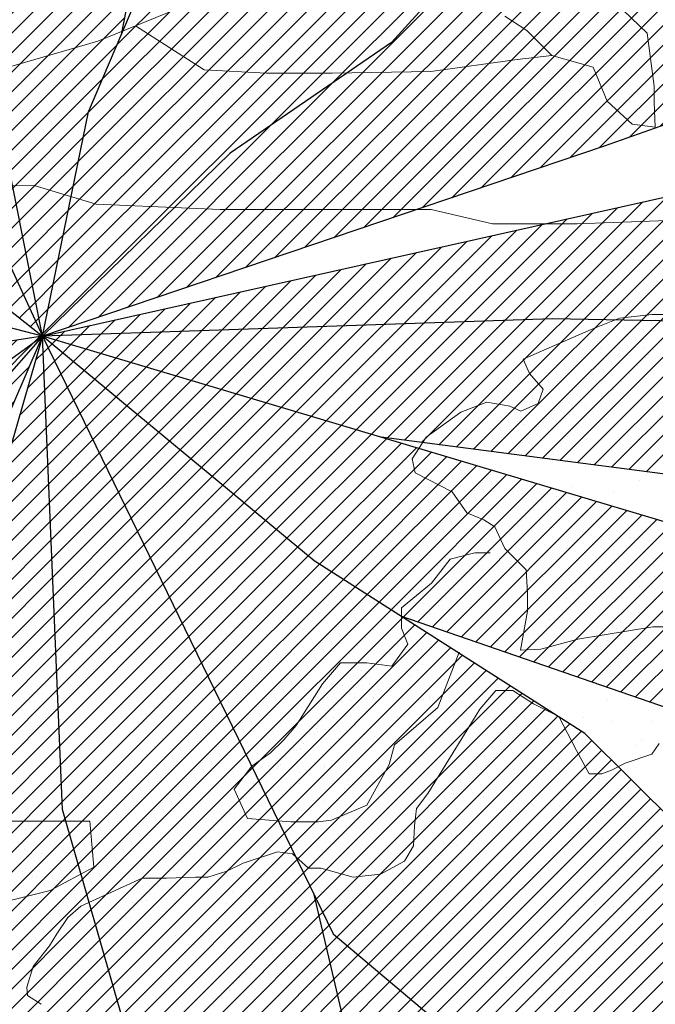
# Model space of a CAD drawing. Units: inches. Extents: x 1986 to 21484, y -1816 to 2016.
# Tile 29 of 85: x 2172.01 to 2179.1, y 1876.39 to 1887.36. Entities that reach past the tile are written whole.
import ezdxf

# ---------------------------------------------------------------- set-up
doc = ezdxf.new("R2010")
doc.units = ezdxf.units.IN
doc.layers.add('L-PLNT', color=84, linetype='Continuous', lineweight=13)
doc.layers.add('vfolhas', color=114, linetype='Continuous', lineweight=5)
for name, color, linetype in [('vfolha', 72, 'Continuous'), ('vfolha2', 110, 'Continuous'), ('vfolhas2', 102, 'Continuous')]:
    doc.layers.add(name, color=color, linetype=linetype)
pattern_1 = [(45, (-2446.5133113, 50.986076), (-0.004419417382, 0.004419417382), [])]

# ---------------------------------------------------------------- blocks, each defined once
blk = doc.blocks.new('arbusto_PB_verde_grande')
at = {"layer": 'vfolha2'}
h = blk.add_hatch(dxfattribs=at)
h.set_pattern_fill('ANSI31', color=256, scale=0.05, style=0)
h.set_pattern_definition(pattern_1)
h.paths.add_polyline_path([(0.02944, 0.35651), (0.00028, 0.09048), (0.02625, -0.03934), (0.047, 0.06233), (0.06189, 0.09731), (0.09372, 0.26573), (0.09955, 0.43473), (0.08789, 0.61313), (0.0645, 0.72266), (0.04988, 0.6851), (0.0236, 0.51294)])
h.paths.add_polyline_path([(0.30106, 0.43789), (0.14225, 0.24871), (0.26685, 0.30022)])
h.paths.add_polyline_path([(0.37995, 0.22817), (0.23697, 0.15193), (0.18428, 0.09364), (0.11122, 0.04358), (0.02625, -0.03934), (0.28061, 0.04667), (0.36829, 0.07798), (0.46756, 0.11239), (0.61068, 0.19376), (0.71585, 0.27823), (0.55813, 0.25948)])
h.paths.add_polyline_path([(0.56101, -0.29441), (0.72752, -0.32573), (0.59024, -0.2412), (0.42962, -0.15982), (0.02625, -0.03934), (0.14922, -0.14107), (0.18838, -0.16604), (0.41501, -0.24435)])
h.paths.add_polyline_path([(-0.27429, -0.44776), (-0.30352, -0.72628), (-0.23923, -0.64175), (-0.15457, -0.45716), (0.02625, -0.03934), (-0.16328, -0.25376)])
h.paths.add_polyline_path([(-0.51963, -0.24744), (-0.67736, -0.32573), (-0.59558, -0.35072), (-0.40574, -0.32882), (-0.21007, -0.20995), (0.02625, -0.03934), (-0.14874, -0.06595), (-0.31518, -0.09101), (-0.41452, -0.15048)])
h.paths.add_polyline_path([(-0.52546, 0.25007), (-0.70947, 0.24698), (-0.51963, 0.1093), (-0.32979, 0.02167), (-0.07567, -0.0128), (-0.04234, -0.02148), (-0.35024, 0.1312)])
h = blk.add_hatch(dxfattribs=at)
h.set_pattern_fill('ANSI31', color=256, scale=0.05, style=0)
h.set_pattern_definition(pattern_1)
h.paths.add_polyline_path([(-0.18963, 0.29704), (-0.08553, 0.20192), (-0.10785, 0.25007), (-0.13202, 0.31865), (-0.25096, 0.48479), (-0.44952, 0.5505), (-0.37946, 0.43789)])
h.paths.add_polyline_path([(0.07911, -0.4071), (0.08214, -0.50631), (0.17255, -0.6355), (0.18428, -0.44151), (0.14904, -0.29177), (0.02625, -0.03934), (0.03527, -0.25376)])
at = {"layer": 'vfolhas'}
h = blk.add_hatch(dxfattribs=at)
h.set_pattern_fill('ANSI31', color=256, scale=0.05, style=0)
h.set_pattern_definition(pattern_1)
h.paths.add_polyline_path([(-0.07279, 0.50669), (-0.18085, 0.65063), (-0.2334, 0.67253), (-0.20712, 0.53176), (-0.10785, 0.25007), (0.02625, -0.03934), (0.00028, 0.09048), (0.00816, 0.16241), (-0.04939, 0.29079)])
h.paths.add_polyline_path([(0.09902, 0.41929), (0.09372, 0.26573), (0.07906, 0.18814), (0.15506, 0.36901), (0.26606, 0.5505), (0.28356, 0.63504), (0.2485, 0.68819), (0.25145, 0.63504), (0.20178, 0.54426)])
h.paths.add_polyline_path([(0.12295, 0.24073), (0.047, 0.06233), (0.02625, -0.03934), (0.11122, 0.04358), (0.18428, 0.09364), (0.27478, 0.19376), (0.3215, 0.25323), (0.44129, 0.38467), (0.47634, 0.57866), (0.41789, 0.45347), (0.28939, 0.30954)])
h.paths.add_polyline_path([(0.58145, -0.03779), (0.70707, 0.01536), (0.78591, 0.04667), (0.74796, 0.06549), (0.62818, 0.08423), (0.52595, 0.09048), (0.39745, 0.04358), (0.02625, -0.03934), (0.25728, -0.03154), (0.43834, -0.0347)])
h.paths.add_polyline_path([(0.52022, -0.03647), (0.43834, -0.0347), (0.25728, -0.03154), (0.02625, -0.03934), (0.17964, -0.08515), (0.53768, -0.13167), (0.69541, -0.15357), (0.78591, -0.07852), (0.70413, -0.10042)])
h.paths.add_polyline_path([(0.27189, -0.21929), (0.14922, -0.14107), (0.02625, -0.03934), (0.15794, -0.31007), (0.29522, -0.42585), (0.41789, -0.49157), (0.56396, -0.56669), (0.5114, -0.48532), (0.39456, -0.34139)])
h.paths.add_polyline_path([(-0.05818, -0.47591), (-0.02312, -0.61984), (0.047, -0.80134), (0.08494, -0.59794), (0.07911, -0.4071), (0.03527, -0.25376), (0.02625, -0.03934), (-0.03773, -0.26001)])
h.paths.add_polyline_path([(-0.24218, 0.14054), (-0.11073, 0.06858), (0.02625, -0.03934), (-0.04235, 0.10871), (-0.21007, 0.23757), (-0.36485, 0.33145), (-0.47874, 0.40341), (-0.54303, 0.46288), (-0.49041, 0.33145), (-0.39408, 0.22192)])
h = blk.add_hatch(dxfattribs=at)
h.set_pattern_fill('ANSI31', color=256, scale=0.05, style=0)
h.set_pattern_definition(pattern_1)
h.paths.add_polyline_path([(-0.57219, 0.06233), (-0.7153, 0.10298), (-0.67736, 0.08107), (-0.62769, 0.01536), (-0.56347, -0.04095), (-0.26461, -0.0834), (-0.14874, -0.06595), (-0.10151, -0.05877), (-0.20418, -0.0472), (-0.40279, -0.00339)])
h.paths.add_polyline_path([(-0.56347, -0.04095), (-0.58279, -0.02401), (-0.72992, -0.09726), (-0.4334, -0.1679), (-0.41452, -0.15048), (-0.31518, -0.09101), (-0.26461, -0.0834)])
h.paths.add_polyline_path([(-0.2769, -0.47267), (-0.27429, -0.44776), (-0.16328, -0.25376), (0.02625, -0.03934), (-0.21007, -0.20995), (-0.2672, -0.24466), (-0.36485, -0.35697), (-0.42907, -0.46341), (-0.47586, -0.60425), (-0.37946, -0.57603)])
h = blk.add_hatch(dxfattribs=at)
h.set_pattern_fill('ANSI31', color=256, scale=0.05, style=0)
h.set_pattern_definition(pattern_1)
h.paths.add_polyline_path([(0.33611, -0.623), (0.43251, -0.67306), (0.39456, -0.59485), (0.3303, -0.44464), (0.29522, -0.42585), (0.15794, -0.31007), (0.14904, -0.29177), (0.18428, -0.44151)])
at = {"layer": 'vfolha'}
for p, q in [((0.02625, -0.03934), (-0.14874, -0.06595)), ((0.02625, -0.03934), (-0.03773, -0.26001)), ((0.03527, -0.25376), (0.02625, -0.03934)), ((0.53768, -0.13167), (0.17964, -0.08515)), ((0.39456, -0.34139), (0.27189, -0.21929)), ((0.07911, -0.4071), (0.03527, -0.25376)), ((0.15794, -0.31007), (0.29522, -0.42585))]:
    blk.add_line(p, q, dxfattribs=at)
at = {"layer": 'vfolha2'}
for p, q in [((0.02625, -0.03934), (0.00028, 0.09048)), ((0.36829, 0.07798), (0.28061, 0.04667)), ((0.28061, 0.04667), (0.02625, -0.03934)), ((-0.21007, -0.20995), (0.02625, -0.03934)), ((0.02625, -0.03934), (-0.16328, -0.25376)), ((-0.15457, -0.45716), (0.02625, -0.03934)), ((0.42962, -0.15982), (0.02625, -0.03934)), ((0.02625, -0.03934), (0.15794, -0.31007)), ((0.18838, -0.16604), (0.41501, -0.24435)), ((0.18428, -0.44151), (0.14904, -0.29177))]:
    blk.add_line(p, q, dxfattribs=at)
at = {"layer": 'vfolhas2'}
for p, q in [((0.09372, 0.26573), (0.06189, 0.09731)), ((-0.10785, 0.25007), (0.02625, -0.03934)), ((0.047, 0.06233), (0.12295, 0.24073)), ((0.27478, 0.19376), (0.18428, 0.09364)), ((0.18428, 0.09364), (0.11122, 0.04358)), ((-0.11073, 0.06858), (0.02625, -0.03934)), ((0.02625, -0.03934), (0.047, 0.06233)), ((0.02625, -0.03934), (0.39745, 0.04358)), ((0.11122, 0.04358), (0.02625, -0.03934)), ((0.02625, -0.03934), (-0.07567, -0.0128)), ((0.25728, -0.03154), (0.02625, -0.03934)), ((0.43834, -0.0347), (0.25728, -0.03154)), ((0.14922, -0.14107), (0.02625, -0.03934)), ((0.27189, -0.21929), (0.14922, -0.14107))]:
    blk.add_line(p, q, dxfattribs=at)
blk = doc.blocks.new('PLANT-SHRUB')
for p, q in [((2172.884, 1887.124), (2174.221, 1887.672)), ((2177.667, 1887.245), (2177.42, 1887.405)), ((2178.739, 1887.472), (2179.007, 1887.215)), ((2173.303, 1887.296), (2174.071, 1886.806)), ((2177.945, 1886.966), (2177.667, 1887.245)), ((2179.007, 1887.215), (2179.086, 1886.623)), ((2171.581, 1886.748), (2172.884, 1887.124)), ((2177.558, 1886.922), (2177.945, 1886.966)), ((2178.404, 1886.835), (2177.945, 1886.966)), ((2176.595, 1886.787), (2177.558, 1886.922)), ((2178.56, 1886.456), (2178.404, 1886.835)), ((2174.071, 1886.806), (2174.764, 1886.768)), ((2174.764, 1886.768), (2175.497, 1886.768)), ((2175.497, 1886.768), (2176.595, 1886.787)), ((2179.086, 1886.623), (2179.086, 1886.444)), ((2178.84, 1886.199), (2178.56, 1886.456)), ((2179.086, 1886.444), (2179.097, 1886.165)), ((2179.097, 1886.165), (2178.84, 1886.199)), ((2179.097, 1886.165), (2179.097, 1886.165)), ((2170.913, 1885.503), (2172.174, 1885.515)), ((2172.174, 1885.515), (2172.865, 1885.309)), ((2172.865, 1885.309), (2174.246, 1885.249)), ((2174.246, 1885.249), (2175.422, 1885.249)), ((2175.422, 1885.249), (2176.598, 1885.249)), ((2176.598, 1885.249), (2177.283, 1885.089)), ((2172.051, 1885.068), (2172.051, 1885.068)), ((2172.187, 1885.064), (2172.187, 1885.064)), ((2177.283, 1885.089), (2178.228, 1885.089)), ((2178.228, 1885.089), (2179.234, 1885.126)), ((2172.457, 1884.857), (2172.457, 1884.857)), ((2172.411, 1884.739), (2172.411, 1884.739)), ((2172.597, 1884.813), (2172.597, 1884.813)), ((2178.584, 1884.814), (2178.584, 1884.814)), ((2172.175, 1884.679), (2172.175, 1884.679)), ((2172.374, 1884.705), (2172.374, 1884.705)), ((2172.714, 1884.659), (2172.714, 1884.659)), ((2178.857, 1884.689), (2178.857, 1884.689)), ((2179.065, 1884.662), (2179.065, 1884.662)), ((2172.175, 1884.523), (2172.175, 1884.523)), ((2172.209, 1884.566), (2172.209, 1884.566)), ((2172.242, 1884.526), (2172.242, 1884.526)), ((2172.294, 1884.62), (2172.294, 1884.62)), ((2172.832, 1884.565), (2172.832, 1884.565)), ((2172.916, 1884.619), (2172.916, 1884.619)), ((2172.974, 1884.53), (2172.974, 1884.53)), ((2173.011, 1884.564), (2173.011, 1884.564)), ((2172.404, 1884.504), (2172.404, 1884.504)), ((2172.444, 1884.472), (2172.444, 1884.472)), ((2172.676, 1884.468), (2172.676, 1884.468)), ((2172.78, 1884.455), (2172.78, 1884.455)), ((2172.942, 1884.433), (2172.942, 1884.433)), ((2172.955, 1884.474), (2172.955, 1884.474)), ((2172.436, 1884.313), (2172.436, 1884.313)), ((2172.776, 1884.348), (2172.776, 1884.348)), ((2178.712, 1884.399), (2178.712, 1884.399)), ((2172.702, 1884.274), (2172.702, 1884.274)), ((2179.06, 1884.079), (2178.7, 1884.036)), ((2178.816, 1884.161), (2178.816, 1884.161)), ((2179.28, 1884.079), (2179.06, 1884.079)), ((2178.7, 1884.036), (2178.383, 1883.913)), ((2178.648, 1884.053), (2178.648, 1884.053)), ((2178.383, 1883.913), (2177.627, 1883.579)), ((2178.489, 1883.703), (2178.489, 1883.703)), ((2178.697, 1883.676), (2178.697, 1883.676)), ((2178.966, 1883.713), (2178.966, 1883.713)), ((2177.627, 1883.579), (2177.697, 1883.42)), ((2178.687, 1883.629), (2178.687, 1883.629)), ((2179.022, 1883.633), (2179.022, 1883.633)), ((2177.697, 1883.42), (2177.847, 1883.245)), ((2178.545, 1883.327), (2178.545, 1883.327)), ((2178.619, 1883.394), (2178.619, 1883.394)), ((2177.847, 1883.245), (2177.794, 1883.087)), ((2178.18, 1883.229), (2178.18, 1883.229)), ((2177.22, 1883.101), (2176.932, 1882.99)), ((2177.476, 1883.057), (2177.22, 1883.101)), ((2178.493, 1883.16), (2178.493, 1883.16)), ((2176.932, 1882.99), (2176.543, 1882.712)), ((2176.932, 1882.99), (2176.932, 1882.99)), ((2177.598, 1883.001), (2177.476, 1883.057)), ((2177.794, 1883.087), (2177.598, 1883.001)), ((2178.325, 1883.052), (2178.325, 1883.052)), ((2178.147, 1882.962), (2178.147, 1882.962)), ((2177.577, 1882.788), (2177.577, 1882.788)), ((2177.639, 1882.854), (2177.639, 1882.854)), ((2178.661, 1882.859), (2178.661, 1882.859)), ((2176.543, 1882.712), (2176.387, 1882.468)), ((2178.12, 1882.717), (2178.12, 1882.717)), ((2178.328, 1882.689), (2178.328, 1882.689)), ((2177.533, 1882.548), (2177.533, 1882.548)), ((2177.726, 1882.576), (2177.726, 1882.576)), ((2177.799, 1882.644), (2177.799, 1882.644)), ((2178.653, 1882.647), (2178.653, 1882.647)), ((2178.777, 1882.546), (2178.777, 1882.546)), ((2176.387, 1882.468), (2176.42, 1882.313)), ((2178.154, 1882.458), (2178.154, 1882.458)), ((2176.42, 1882.313), (2176.832, 1882.102)), ((2177.328, 1882.212), (2177.328, 1882.212)), ((2178.927, 1882.225), (2178.927, 1882.225)), ((2179.001, 1882.293), (2179.001, 1882.293)), ((2176.832, 1882.102), (2176.998, 1881.869)), ((2176.926, 1882.161), (2176.926, 1882.161)), ((2178.171, 1882.159), (2178.171, 1882.159)), ((2177.614, 1882.084), (2177.614, 1882.084)), ((2178.002, 1882.052), (2178.002, 1882.052)), ((2178.636, 1882.089), (2178.636, 1882.089)), ((2176.998, 1881.869), (2177.187, 1881.791)), ((2177.187, 1881.791), (2177.309, 1881.713)), ((2178.529, 1881.861), (2178.529, 1881.861)), ((2177.309, 1881.713), (2177.42, 1881.469)), ((2177.309, 1881.713), (2177.309, 1881.713)), ((2177.752, 1881.731), (2177.752, 1881.731)), ((2177.96, 1881.703), (2177.96, 1881.703)), ((2178.129, 1881.688), (2178.129, 1881.688)), ((2178.285, 1881.66), (2178.285, 1881.66)), ((2178.827, 1881.589), (2178.827, 1881.589)), ((2179.036, 1881.561), (2179.036, 1881.561)), ((2177.42, 1881.469), (2177.66, 1881.234)), ((2178.108, 1881.475), (2178.108, 1881.475)), ((2178.182, 1881.542), (2178.182, 1881.542)), ((2178.455, 1881.545), (2178.455, 1881.545)), ((2176.812, 1881.351), (2176.604, 1881.085)), ((2177.088, 1881.42), (2176.812, 1881.351)), ((2177.256, 1881.42), (2177.088, 1881.42)), ((2177.589, 1881.314), (2177.589, 1881.314)), ((2177.66, 1881.234), (2177.672, 1880.972)), ((2178.611, 1881.319), (2178.611, 1881.319)), ((2177.848, 1881.158), (2177.848, 1881.158)), ((2179.092, 1881.156), (2179.092, 1881.156)), ((2176.604, 1881.085), (2176.269, 1880.809)), ((2177.679, 1881.051), (2177.679, 1881.051)), ((2177.71, 1881.11), (2177.71, 1881.11)), ((2178.924, 1881.049), (2178.924, 1881.049)), ((2176.53, 1880.942), (2176.53, 1880.942)), ((2177.672, 1880.972), (2177.672, 1880.772)), ((2178.104, 1880.918), (2178.104, 1880.918)), ((2176.269, 1880.809), (2176.269, 1880.582)), ((2176.284, 1880.801), (2176.284, 1880.801)), ((2176.411, 1880.872), (2176.411, 1880.872)), ((2176.515, 1880.858), (2176.515, 1880.858)), ((2176.678, 1880.837), (2176.678, 1880.837)), ((2176.735, 1880.717), (2176.735, 1880.717)), ((2177.672, 1880.772), (2177.597, 1880.335)), ((2177.916, 1880.674), (2177.916, 1880.674)), ((2178.912, 1880.76), (2178.912, 1880.76)), ((2176.269, 1880.582), (2176.338, 1880.404)), ((2176.603, 1880.606), (2176.603, 1880.606)), ((2178.234, 1880.46), (2179.071, 1880.597)), ((2178.459, 1880.603), (2178.459, 1880.603)), ((2178.667, 1880.575), (2178.667, 1880.575)), ((2179.071, 1880.597), (2179.221, 1880.597)), ((2176.517, 1880.557), (2176.517, 1880.557)), ((2176.519, 1880.553), (2176.519, 1880.553)), ((2176.524, 1880.524), (2176.524, 1880.524)), ((2176.561, 1880.558), (2176.561, 1880.558)), ((2177.822, 1880.348), (2178.234, 1880.46)), ((2178.132, 1880.544), (2178.132, 1880.544)), ((2178.234, 1880.46), (2178.234, 1880.46)), ((2178.586, 1880.548), (2178.586, 1880.548)), ((2178.992, 1880.532), (2178.992, 1880.532)), ((2176.338, 1880.404), (2176.16, 1880.158)), ((2176.331, 1880.365), (2176.331, 1880.365)), ((2176.758, 1880.372), (2176.758, 1880.372)), ((2177.597, 1880.335), (2177.822, 1880.348)), ((2178.49, 1880.373), (2178.49, 1880.373)), ((2178.564, 1880.441), (2178.564, 1880.441)), ((2176.325, 1880.342), (2176.325, 1880.342)), ((2176.494, 1880.344), (2176.494, 1880.344)), ((2176.674, 1879.698), (2176.912, 1880.313)), ((2176.745, 1880.299), (2176.745, 1880.299)), ((2176.765, 1880.308), (2176.765, 1880.308)), ((2176.869, 1880.295), (2176.869, 1880.295)), ((2175.588, 1880.197), (2175.39, 1879.961)), ((2175.884, 1880.197), (2175.588, 1880.197)), ((2176.16, 1880.158), (2175.884, 1880.197)), ((2176.115, 1880.149), (2176.115, 1880.149)), ((2176.505, 1880.172), (2176.505, 1880.172)), ((2178.079, 1880.148), (2178.079, 1880.148)), ((2178.77, 1880.155), (2178.77, 1880.155)), ((2175.735, 1880.053), (2175.735, 1880.053)), ((2175.82, 1880.107), (2175.82, 1880.107)), ((2176.358, 1880.052), (2176.358, 1880.052)), ((2176.442, 1880.106), (2176.442, 1880.106)), ((2178.601, 1880.048), (2178.601, 1880.048)), ((2175.39, 1879.961), (2175.094, 1879.497)), ((2175.505, 1879.957), (2175.505, 1879.957)), ((2175.609, 1879.943), (2175.609, 1879.943)), ((2175.711, 1879.991), (2175.711, 1879.991)), ((2175.771, 1879.922), (2175.771, 1879.922)), ((2175.916, 1879.967), (2175.916, 1879.967)), ((2176.235, 1879.985), (2176.235, 1879.985)), ((2176.715, 1879.974), (2176.715, 1879.974)), ((2176.746, 1879.987), (2176.746, 1879.987)), ((2176.752, 1880.007), (2176.752, 1880.007)), ((2178.092, 1880.009), (2178.092, 1880.009)), ((2175.339, 1879.801), (2175.339, 1879.801)), ((2175.441, 1879.804), (2175.441, 1879.804)), ((2175.742, 1879.807), (2175.742, 1879.807)), ((2175.952, 1879.806), (2175.952, 1879.806)), ((2175.962, 1879.8), (2175.962, 1879.8)), ((2176.043, 1879.886), (2176.043, 1879.886)), ((2176.147, 1879.872), (2176.147, 1879.872)), ((2176.309, 1879.851), (2176.309, 1879.851)), ((2176.581, 1879.815), (2176.581, 1879.815)), ((2176.584, 1879.799), (2176.584, 1879.799)), ((2176.685, 1879.801), (2176.685, 1879.801)), ((2177.321, 1879.888), (2177.141, 1879.678)), ((2177.511, 1879.888), (2177.321, 1879.888)), ((2177.741, 1879.738), (2177.511, 1879.888)), ((2175.705, 1879.774), (2175.705, 1879.774)), ((2176.19, 1879.28), (2176.674, 1879.698)), ((2176.492, 1879.787), (2176.492, 1879.787)), ((2176.516, 1879.791), (2176.516, 1879.791)), ((2178.021, 1879.598), (2177.741, 1879.738)), ((2178.561, 1879.778), (2178.561, 1879.778)), ((2175.506, 1879.591), (2175.506, 1879.591)), ((2175.658, 1879.607), (2175.658, 1879.607)), ((2175.699, 1879.606), (2175.699, 1879.606)), ((2176.222, 1879.599), (2176.222, 1879.599)), ((2176.28, 1879.606), (2176.28, 1879.606)), ((2176.306, 1879.598), (2176.306, 1879.598)), ((2176.343, 1879.632), (2176.343, 1879.632)), ((2177.141, 1879.678), (2177.02, 1879.478)), ((2178.021, 1879.598), (2178.021, 1879.598)), ((2178.221, 1879.219), (2178.021, 1879.598)), ((2178.091, 1879.616), (2178.091, 1879.616)), ((2178.299, 1879.589), (2178.299, 1879.589)), ((2175.094, 1879.497), (2174.956, 1879.339)), ((2175.574, 1879.553), (2175.574, 1879.553)), ((2176.196, 1879.552), (2176.196, 1879.552)), ((2177.02, 1879.478), (2176.561, 1878.739)), ((2177.02, 1879.478), (2177.02, 1879.478)), ((2177.809, 1879.543), (2177.809, 1879.543)), ((2178.623, 1879.546), (2178.623, 1879.546)), ((2179.054, 1879.541), (2179.054, 1879.541)), ((2175.295, 1879.398), (2175.295, 1879.398)), ((2175.321, 1879.464), (2175.321, 1879.464)), ((2175.332, 1879.432), (2175.332, 1879.432)), ((2175.425, 1879.45), (2175.425, 1879.45)), ((2175.429, 1879.419), (2175.429, 1879.419)), ((2175.587, 1879.428), (2175.587, 1879.428)), ((2175.859, 1879.393), (2175.859, 1879.393)), ((2175.94, 1879.421), (2175.94, 1879.421)), ((2175.963, 1879.379), (2175.963, 1879.379)), ((2176.107, 1879.416), (2176.107, 1879.416)), ((2176.125, 1879.358), (2176.125, 1879.358)), ((2178.054, 1879.378), (2178.054, 1879.378)), ((2174.956, 1879.339), (2174.808, 1879.191)), ((2175.178, 1879.301), (2175.178, 1879.301)), ((2175.8, 1879.3), (2175.8, 1879.3)), ((2175.933, 1879.257), (2175.933, 1879.257)), ((2176.131, 1879.063), (2176.19, 1879.28)), ((2177.273, 1879.258), (2177.273, 1879.258)), ((2178.873, 1879.272), (2178.873, 1879.272)), ((2178.946, 1879.34), (2178.946, 1879.34)), ((2179.141, 1879.298), (2179.061, 1879.179)), ((2174.808, 1879.191), (2174.601, 1879.043)), ((2175.097, 1879.216), (2175.097, 1879.216)), ((2175.147, 1879.241), (2175.147, 1879.241)), ((2175.686, 1879.221), (2175.686, 1879.221)), ((2175.896, 1879.223), (2175.896, 1879.223)), ((2177.202, 1879.157), (2177.202, 1879.157)), ((2178.221, 1879.219), (2178.221, 1879.219)), ((2178.361, 1878.959), (2178.221, 1879.219)), ((2178.447, 1879.154), (2178.447, 1879.154)), ((2179.061, 1879.179), (2178.761, 1879.079)), ((2174.601, 1879.043), (2174.403, 1878.787)), ((2174.703, 1879.028), (2174.703, 1879.028)), ((2174.79, 1879.054), (2174.79, 1879.054)), ((2174.874, 1879.107), (2174.874, 1879.107)), ((2174.893, 1879.04), (2174.893, 1879.04)), ((2174.923, 1879.057), (2174.923, 1879.057)), ((2175.413, 1879.053), (2175.413, 1879.053)), ((2175.416, 1879.034), (2175.416, 1879.034)), ((2175.497, 1879.106), (2175.497, 1879.106)), ((2175.697, 1879.041), (2175.697, 1879.041)), ((2175.884, 1878.61), (2176.131, 1879.063)), ((2175.927, 1879.036), (2175.927, 1879.036)), ((2176.035, 1879.051), (2176.035, 1879.051)), ((2176.119, 1879.105), (2176.119, 1879.105)), ((2177.034, 1879.049), (2177.034, 1879.049)), ((2178.278, 1879.047), (2178.278, 1879.047)), ((2178.761, 1879.079), (2178.611, 1878.999)), ((2174.865, 1879.006), (2174.865, 1879.006)), ((2174.886, 1879.023), (2174.886, 1879.023)), ((2175.136, 1878.97), (2175.136, 1878.97)), ((2175.24, 1878.957), (2175.24, 1878.957)), ((2175.403, 1878.935), (2175.403, 1878.935)), ((2176.926, 1878.94), (2176.926, 1878.94)), ((2177.513, 1879.003), (2177.513, 1879.003)), ((2178.501, 1878.959), (2178.361, 1878.959)), ((2178.611, 1878.999), (2178.501, 1878.959)), ((2178.536, 1879.008), (2178.536, 1879.008)), ((2174.623, 1878.853), (2174.623, 1878.853)), ((2174.687, 1878.841), (2174.687, 1878.841)), ((2175.134, 1878.855), (2175.134, 1878.855)), ((2175.487, 1878.848), (2175.487, 1878.848)), ((2175.523, 1878.881), (2175.523, 1878.881)), ((2175.674, 1878.9), (2175.674, 1878.9)), ((2175.674, 1878.836), (2175.674, 1878.836)), ((2175.778, 1878.886), (2175.778, 1878.886)), ((2175.941, 1878.864), (2175.941, 1878.864)), ((2176.852, 1878.872), (2176.852, 1878.872)), ((2178.475, 1878.907), (2178.475, 1878.907)), ((2174.403, 1878.787), (2174.552, 1878.462)), ((2175.016, 1878.8), (2175.016, 1878.8)), ((2175.639, 1878.799), (2175.639, 1878.799)), ((2176.561, 1878.739), (2176.437, 1878.57)), ((2176.646, 1878.772), (2176.646, 1878.772)), ((2176.854, 1878.744), (2176.854, 1878.744)), ((2177.179, 1878.701), (2177.179, 1878.701)), ((2174.476, 1878.648), (2174.476, 1878.648)), ((2174.513, 1878.681), (2174.513, 1878.681)), ((2174.713, 1878.607), (2174.713, 1878.607)), ((2174.88, 1878.655), (2174.88, 1878.655)), ((2175.288, 1878.665), (2175.288, 1878.665)), ((2175.335, 1878.606), (2175.335, 1878.606)), ((2175.403, 1878.649), (2175.403, 1878.649)), ((2175.489, 1878.442), (2175.884, 1878.61)), ((2176.949, 1878.647), (2176.949, 1878.647)), ((2177.722, 1878.63), (2177.722, 1878.63)), ((2177.93, 1878.603), (2177.93, 1878.603)), ((2178.028, 1878.608), (2178.028, 1878.608)), ((2178.127, 1878.589), (2178.127, 1878.589)), ((2179.075, 1878.595), (2179.075, 1878.595)), ((2174.629, 1878.553), (2174.629, 1878.553)), ((2174.681, 1878.513), (2174.681, 1878.513)), ((2175.114, 1878.506), (2175.114, 1878.506)), ((2175.251, 1878.552), (2175.251, 1878.552)), ((2176.437, 1878.57), (2176.415, 1878.379)), ((2176.454, 1878.508), (2176.454, 1878.508)), ((2177.486, 1878.542), (2177.486, 1878.542)), ((2178.053, 1878.521), (2178.053, 1878.521)), ((2178.255, 1878.56), (2178.255, 1878.56)), ((2178.731, 1878.54), (2178.731, 1878.54)), ((2178.798, 1878.488), (2178.798, 1878.488)), ((2171.534, 1878.429), (2172.793, 1878.429)), ((2172.793, 1878.429), (2172.84, 1877.916)), ((2174.552, 1878.462), (2175.035, 1878.422)), ((2174.61, 1878.468), (2174.61, 1878.468)), ((2174.952, 1878.477), (2174.952, 1878.477)), ((2175.035, 1878.422), (2175.341, 1878.422)), ((2175.056, 1878.464), (2175.056, 1878.464)), ((2175.077, 1878.472), (2175.077, 1878.472)), ((2175.121, 1878.47), (2175.121, 1878.47)), ((2175.219, 1878.442), (2175.219, 1878.442)), ((2175.341, 1878.422), (2175.489, 1878.442)), ((2176.415, 1878.379), (2176.404, 1878.154)), ((2179.006, 1878.461), (2179.006, 1878.461)), ((2172.078, 1878.338), (2172.078, 1878.338)), ((2172.182, 1878.324), (2172.182, 1878.324)), ((2172.243, 1878.311), (2172.243, 1878.311)), ((2172.345, 1878.303), (2172.345, 1878.303)), ((2172.366, 1878.304), (2172.366, 1878.304)), ((2172.492, 1878.282), (2172.492, 1878.282)), ((2172.616, 1878.267), (2172.616, 1878.267)), ((2172.754, 1878.313), (2172.754, 1878.313)), ((2172.456, 1878.248), (2172.456, 1878.248)), ((2172.72, 1878.254), (2172.72, 1878.254)), ((2176.404, 1878.154), (2176.302, 1877.986)), ((2176.442, 1878.247), (2176.442, 1878.247)), ((2176.879, 1878.156), (2176.879, 1878.156)), ((2177.488, 1878.233), (2177.488, 1878.233)), ((2177.656, 1878.157), (2177.656, 1878.157)), ((2178.124, 1878.154), (2178.124, 1878.154)), ((2178.51, 1878.238), (2178.51, 1878.238)), ((2172.062, 1878.111), (2172.062, 1878.111)), ((2172.257, 1878.066), (2172.257, 1878.066)), ((2172.5, 1878.113), (2172.5, 1878.113)), ((2172.6, 1878.056), (2172.6, 1878.056)), ((2172.685, 1878.11), (2172.685, 1878.11)), ((2174.885, 1878.087), (2174.503, 1877.963)), ((2175.054, 1878.065), (2174.885, 1878.087)), ((2175.011, 1878.05), (2175.011, 1878.05)), ((2175.054, 1878.065), (2175.054, 1878.065)), ((2175.234, 1877.907), (2175.054, 1878.065)), ((2176.711, 1878.048), (2176.711, 1878.048)), ((2177.956, 1878.046), (2177.956, 1878.046)), ((2174.503, 1877.963), (2174.323, 1877.874)), ((2174.543, 1877.967), (2174.543, 1877.967)), ((2174.88, 1877.956), (2174.88, 1877.956)), ((2174.961, 1877.962), (2174.961, 1877.962)), ((2176.302, 1877.986), (2176.033, 1877.84)), ((2172.046, 1877.872), (2172.046, 1877.872)), ((2172.083, 1877.906), (2172.083, 1877.906)), ((2172.23, 1877.926), (2172.23, 1877.926)), ((2172.84, 1877.916), (2172.352, 1877.656)), ((2172.741, 1877.928), (2172.741, 1877.928)), ((2172.84, 1877.916), (2172.84, 1877.916)), ((2174.323, 1877.874), (2174.109, 1877.806)), ((2174.26, 1877.844), (2174.26, 1877.844)), ((2174.323, 1877.874), (2174.323, 1877.874)), ((2174.39, 1877.827), (2174.39, 1877.827)), ((2174.701, 1877.852), (2174.701, 1877.852)), ((2174.741, 1877.829), (2174.741, 1877.829)), ((2174.768, 1877.895), (2174.768, 1877.895)), ((2175.199, 1877.851), (2175.199, 1877.851)), ((2175.369, 1877.907), (2175.234, 1877.907)), ((2175.266, 1877.894), (2175.266, 1877.894)), ((2175.729, 1877.806), (2175.369, 1877.907)), ((2176.033, 1877.84), (2175.729, 1877.806)), ((2176.924, 1877.877), (2176.924, 1877.877)), ((2177.308, 1877.838), (2177.308, 1877.838)), ((2178.003, 1877.838), (2178.003, 1877.838)), ((2179.049, 1877.825), (2179.049, 1877.825)), ((2172.161, 1877.81), (2172.161, 1877.81)), ((2172.204, 1877.804), (2172.204, 1877.804)), ((2172.432, 1877.774), (2172.432, 1877.774)), ((2172.536, 1877.761), (2172.536, 1877.761)), ((2173.378, 1877.795), (2172.693, 1877.482)), ((2173.378, 1877.795), (2173.378, 1877.795)), ((2173.648, 1877.795), (2173.378, 1877.795)), ((2173.974, 1877.806), (2173.648, 1877.795)), ((2174.109, 1877.806), (2173.974, 1877.806)), ((2174.071, 1877.796), (2174.071, 1877.796)), ((2174.327, 1877.817), (2174.327, 1877.817)), ((2174.607, 1877.798), (2174.607, 1877.798)), ((2174.691, 1877.787), (2174.691, 1877.787)), ((2174.711, 1877.802), (2174.711, 1877.802)), ((2174.736, 1877.819), (2174.736, 1877.819)), ((2174.821, 1877.77), (2174.821, 1877.77)), ((2175.038, 1877.742), (2175.038, 1877.742)), ((2175.121, 1877.731), (2175.121, 1877.731)), ((2175.168, 1877.804), (2175.168, 1877.804)), ((2175.251, 1877.714), (2175.251, 1877.714)), ((2175.36, 1877.816), (2175.36, 1877.816)), ((2175.586, 1877.798), (2175.586, 1877.798)), ((2176.278, 1877.785), (2176.278, 1877.785)), ((2176.486, 1877.758), (2176.486, 1877.758)), ((2176.811, 1877.715), (2176.811, 1877.715)), ((2177.234, 1877.771), (2177.234, 1877.771)), ((2178.857, 1877.806), (2178.857, 1877.806)), ((2172.352, 1877.656), (2171.755, 1877.508)), ((2174.101, 1877.675), (2174.101, 1877.675)), ((2174.384, 1877.65), (2174.384, 1877.65)), ((2174.533, 1877.659), (2174.533, 1877.659)), ((2174.552, 1877.656), (2174.552, 1877.656)), ((2174.882, 1877.65), (2174.882, 1877.65)), ((2174.951, 1877.654), (2174.951, 1877.654)), ((2175.192, 1877.661), (2175.192, 1877.661)), ((2175.221, 1877.688), (2175.221, 1877.688)), ((2175.36, 1877.656), (2175.36, 1877.656)), ((2175.38, 1877.649), (2175.38, 1877.649)), ((2175.468, 1877.685), (2175.468, 1877.685)), ((2175.551, 1877.674), (2175.551, 1877.674)), ((2175.681, 1877.657), (2175.681, 1877.657)), ((2177.354, 1877.644), (2177.354, 1877.644)), ((2177.562, 1877.616), (2177.562, 1877.616)), ((2173.269, 1877.524), (2173.269, 1877.524)), ((2173.429, 1877.548), (2173.429, 1877.548)), ((2174.317, 1877.509), (2174.317, 1877.509)), ((2174.383, 1877.501), (2174.383, 1877.501)), ((2174.413, 1877.528), (2174.413, 1877.528)), ((2174.639, 1877.495), (2174.639, 1877.495)), ((2174.726, 1877.511), (2174.726, 1877.511)), ((2175.033, 1877.515), (2175.033, 1877.515)), ((2175.137, 1877.494), (2175.137, 1877.494)), ((2175.157, 1877.495), (2175.157, 1877.495)), ((2175.919, 1877.544), (2175.919, 1877.544)), ((2177.163, 1877.542), (2177.163, 1877.542)), ((2177.886, 1877.574), (2177.886, 1877.574)), ((2178.408, 1877.539), (2178.408, 1877.539)), ((2178.429, 1877.502), (2178.429, 1877.502)), ((2172.693, 1877.482), (2172.551, 1877.356)), ((2174.46, 1877.404), (2174.46, 1877.404)), ((2174.543, 1877.393), (2174.543, 1877.393)), ((2174.572, 1877.452), (2174.572, 1877.452)), ((2174.894, 1877.388), (2174.894, 1877.388)), ((2175.07, 1877.451), (2175.07, 1877.451)), ((2176.417, 1877.477), (2176.417, 1877.477)), ((2176.836, 1877.406), (2176.836, 1877.406)), ((2177.463, 1877.463), (2177.463, 1877.463)), ((2178.436, 1877.42), (2178.436, 1877.42)), ((2178.485, 1877.468), (2178.485, 1877.468)), ((2178.509, 1877.487), (2178.509, 1877.487)), ((2178.637, 1877.475), (2178.637, 1877.475)), ((2178.962, 1877.432), (2178.962, 1877.432)), ((2172.551, 1877.356), (2172.425, 1877.174)), ((2173.614, 1877.357), (2173.614, 1877.357)), ((2174.523, 1877.351), (2174.523, 1877.351)), ((2174.673, 1877.376), (2174.673, 1877.376)), ((2174.864, 1877.361), (2174.864, 1877.361)), ((2174.89, 1877.347), (2174.89, 1877.347)), ((2174.941, 1877.346), (2174.941, 1877.346)), ((2174.974, 1877.336), (2174.974, 1877.336)), ((2175.104, 1877.319), (2175.104, 1877.319)), ((2172.425, 1877.174), (2172.346, 1877.04)), ((2172.682, 1877.224), (2172.682, 1877.224)), ((2172.823, 1877.162), (2172.823, 1877.162)), ((2172.89, 1877.197), (2172.89, 1877.197)), ((2174.705, 1877.215), (2174.705, 1877.215)), ((2174.716, 1877.203), (2174.716, 1877.203)), ((2174.753, 1877.249), (2174.753, 1877.249)), ((2172.654, 1877.054), (2172.654, 1877.054)), ((2172.728, 1877.149), (2172.728, 1877.149)), ((2173.215, 1877.154), (2173.215, 1877.154)), ((2173.751, 1877.154), (2173.751, 1877.154)), ((2173.758, 1877.082), (2173.758, 1877.082)), ((2173.899, 1877.052), (2173.899, 1877.052)), ((2173.966, 1877.055), (2173.966, 1877.055)), ((2174.067, 1877.159), (2174.067, 1877.159)), ((2174.83, 1877.115), (2174.83, 1877.115)), ((2175.312, 1877.157), (2175.312, 1877.157)), ((2175.876, 1877.102), (2175.876, 1877.102)), ((2176.489, 1877.088), (2176.489, 1877.088)), ((2176.557, 1877.155), (2176.557, 1877.155)), ((2176.899, 1877.107), (2176.899, 1877.107)), ((2177.801, 1877.153), (2177.801, 1877.153)), ((2177.978, 1877.068), (2177.978, 1877.068)), ((2178.038, 1877.055), (2178.038, 1877.055)), ((2179.024, 1877.054), (2179.024, 1877.054)), ((2179.046, 1877.15), (2179.046, 1877.15)), ((2172.346, 1877.04), (2172.164, 1876.811)), ((2173.193, 1876.971), (2173.193, 1876.971)), ((2173.267, 1877.039), (2173.267, 1877.039)), ((2174.291, 1877.012), (2174.291, 1877.012)), ((2174.816, 1877.006), (2174.816, 1877.006)), ((2175.143, 1877.05), (2175.143, 1877.05)), ((2176.388, 1877.048), (2176.388, 1877.048)), ((2176.415, 1877.02), (2176.415, 1877.02)), ((2177.633, 1877.045), (2177.633, 1877.045)), ((2178.877, 1877.043), (2178.877, 1877.043)), ((2174.833, 1876.941), (2174.833, 1876.941)), ((2175.041, 1876.913), (2175.041, 1876.913)), ((2175.366, 1876.871), (2175.366, 1876.871)), ((2172.164, 1876.811), (2172.093, 1876.582)), ((2173.243, 1876.754), (2173.243, 1876.754)), ((2174.29, 1876.74), (2174.29, 1876.74)), ((2175.312, 1876.745), (2175.312, 1876.745)), ((2175.909, 1876.799), (2175.909, 1876.799)), ((2176.117, 1876.772), (2176.117, 1876.772)), ((2176.442, 1876.729), (2176.442, 1876.729)), ((2177.69, 1876.737), (2177.69, 1876.737)), ((2174.394, 1876.62), (2174.394, 1876.62)), ((2174.468, 1876.688), (2174.468, 1876.688)), ((2176.017, 1876.656), (2176.017, 1876.656)), ((2176.391, 1876.706), (2176.391, 1876.706)), ((2176.985, 1876.657), (2176.985, 1876.657)), ((2177.193, 1876.63), (2177.193, 1876.63)), ((2177.438, 1876.693), (2177.438, 1876.693)), ((2177.616, 1876.669), (2177.616, 1876.669)), ((2178.46, 1876.698), (2178.46, 1876.698)), ((2172.093, 1876.582), (2172.101, 1876.487)), ((2172.795, 1876.606), (2172.795, 1876.606)), ((2173.107, 1876.547), (2173.107, 1876.547)), ((2174.351, 1876.545), (2174.351, 1876.545)), ((2175.596, 1876.543), (2175.596, 1876.543)), ((2176.841, 1876.541), (2176.841, 1876.541)), ((2177.518, 1876.587), (2177.518, 1876.587)), ((2178.061, 1876.516), (2178.061, 1876.516)), ((2178.085, 1876.538), (2178.085, 1876.538)), ((2172.101, 1876.487), (2172.251, 1876.392)), ((2178.269, 1876.488), (2178.269, 1876.488)), ((2178.594, 1876.446), (2178.594, 1876.446))]:
    blk.add_line(p, q)

msp = doc.modelspace()

# ---------------------------------------------------------------- block references
at = {"layer": 'L-PLNT'}
msp.add_blockref('PLANT-SHRUB', (0, 0), dxfattribs=at)
at = {"layer": 'L-PLNT', "xscale": 24.60366729364114, "yscale": 24.60366729364114, "zscale": 24.60366729364114}
msp.add_blockref('arbusto_PB_verde_grande', (2171.623, 1884.805), dxfattribs=at)

doc.saveas('drawing.dxf')
